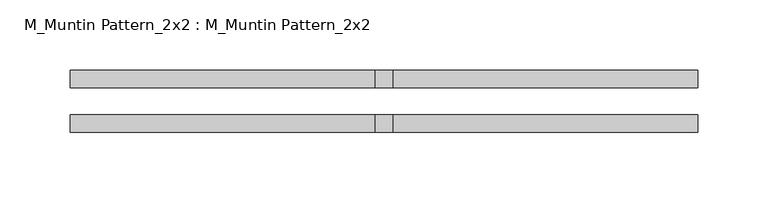
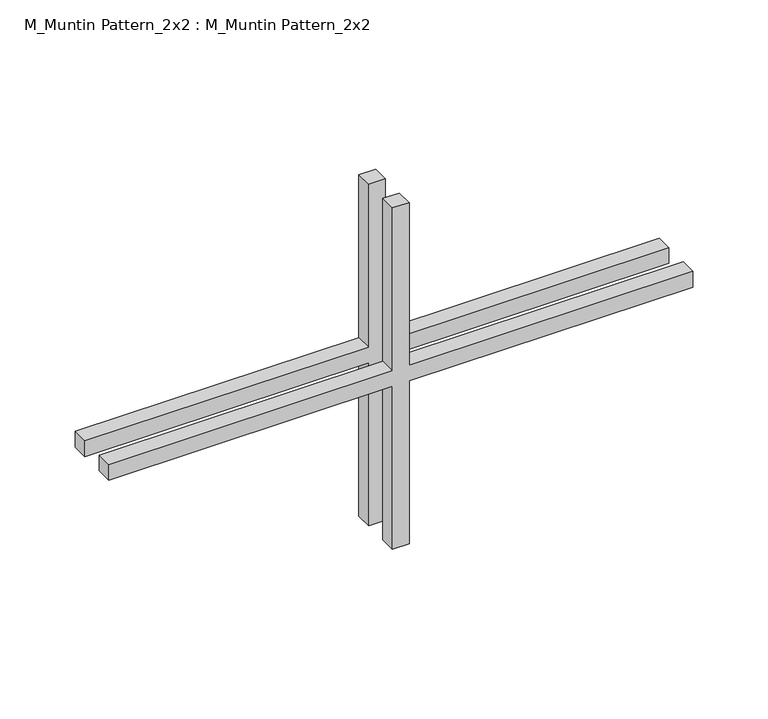
"""IFC4 building model written with IfcOpenShell, lengths in millimetres: proxy geometry, M_Muntin Pattern_2x2 : M_Muntin Pattern_2x2."""

from ifc_helpers import new_model, si_unit, frame, origin, place, context, project, spatial, polyline, outline, extrude, source, transform, mapped, element, save


def m_muntin_pattern_2x2_m_muntin_pattern_2x2_b5651a11(model_context):
    return source(origin(), model_context, "Body", "SweptSolid", [
        extrude(outline(polyline([(144.6375, -6.35), (144.6375, -223.8), (131.9375, -223.8), (131.9375, -6.35), (0.0, -6.35), (0.0, 6.35), (131.9375, 6.35), (131.9375, 223.8), (144.6375, 223.8), (144.6375, 6.35), (276.575, 6.35), (276.575, -6.35), (144.6375, -6.35)])), frame((0.0, 9.525, 0.0), z_axis=(0.0, 1.0, 0.0), x_axis=(0.0, 0.0, 1.0)), (0.0, 0.0, 1.0), 12.7),
        extrude(outline(polyline([(144.6375, -6.35), (144.6375, -223.8), (131.9375, -223.8), (131.9375, -6.35), (0.0, -6.35), (0.0, 6.35), (131.9375, 6.35), (131.9375, 223.8), (144.6375, 223.8), (144.6375, 6.35), (276.575, 6.35), (276.575, -6.35), (144.6375, -6.35)])), frame((0.0, -22.225, 0.0), z_axis=(0.0, 1.0, 0.0), x_axis=(0.0, 0.0, 1.0)), (0.0, 0.0, 1.0), 12.7),
    ])


if __name__ == "__main__":
    model = new_model("IFC4")
    model_context = context("Model", 3, world=origin())
    ifc_project = project(units=[si_unit("LENGTHUNIT", "METRE", prefix="MILLI")], contexts=[model_context])
    site = spatial("IfcSite", under=ifc_project)
    building = spatial("IfcBuilding", under=site)
    placement = place(None, origin())
    m_muntin_pattern_2x2_m_muntin_pattern_2x2_shape = m_muntin_pattern_2x2_m_muntin_pattern_2x2_b5651a11(model_context)
    element("IfcBuildingElementProxy", 1, Name="M_Muntin Pattern_2x2 : M_Muntin Pattern_2x2", ObjectType="M_Muntin Pattern_2x2 : M_Muntin Pattern_2x2", at=placement, inside=building, context=model_context, shape_type="MappedRepresentation", body=[
        mapped(m_muntin_pattern_2x2_m_muntin_pattern_2x2_shape, transform((0.0, 0.0, 0.0), x_axis=(1.0, 0.0, 0.0), y_axis=(0.0, 1.0, 0.0), z_axis=(0.0, 0.0, 1.0))),
    ])
    save(model, "model.ifc")

# Revit data of these elements
# Type "M_Muntin Pattern_2x2 : M_Muntin Pattern_2x2"
#   Width [instance default] = 1.2 m
#   Thickness = 0.0127 m
#   Height [instance default] = 1.2 m
#   Distance = 0.01905 m
#   Interior Material [instance default] = none
#   Exterior Material [instance default] = none
#   Default Elevation = 0
# Element 1 (IfcBuildingElementProxy, "M_Muntin Pattern_2x2 : M_Muntin Pattern_2x2")
#   Width = 0.4476 m
#   Height = 0.276575 m
#   Interior Material = Wood - Stained
#   Exterior Material = Clad - White
#   Materials on its faces: "Clad - White", "Wood - Stained"
# Materials
#   "Clad - White": class "Wood", colour RGB 242 242 238, transparency 0, Cost = 0
#   "Wood - Stained": class "Wood", colour RGB 224 178 126, transparency 0, Cost = 0
